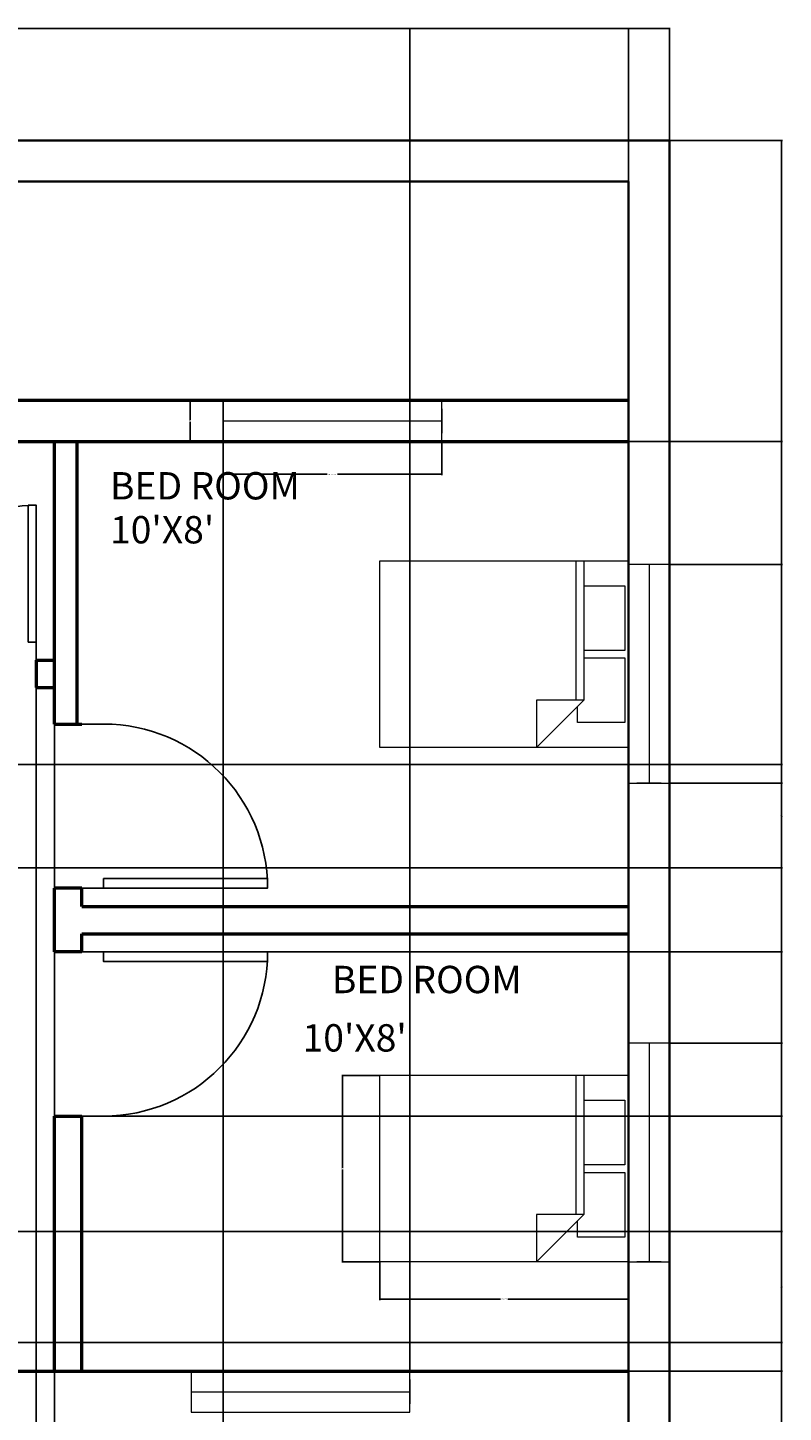
# Model space of a CAD drawing. Units: inches. Extents: x 8049 to 8459, y 820 to 1350.
# Tile 25 of 25: x 8294 to 8459, y 1046 to 1350. Entities that reach past the tile are written whole.
import ezdxf

# ---------------------------------------------------------------- set-up
doc = ezdxf.new("R2010")
doc.units = ezdxf.units.IN
doc.header["$MEASUREMENT"] = 0
for name, color, linetype, lineweight in [('A-ANNO-DIMS', 2, 'Continuous', 18), ('A-AREA-IDEN', 7, 'Continuous', 25), ('A-DOOR', 3, 'Continuous', 25), ('A-FURN', 8, 'Continuous', 18), ('A-GLAZ', 4, 'Continuous', 18), ('A-WALL', 7, 'Continuous', 50), ('C-SITE-WALL', 7, 'Continuous', 35)]:
    doc.layers.add(name, color=color, linetype=linetype, lineweight=lineweight)
doc.styles.get("Standard").update_dxf_attribs({"font": 'arial.ttf'})
doc.dimstyles.get("Standard").update_dxf_attribs({"dimtxt": 0.18, "dimasz": 0.18, "dimexe": 0.18, "dimexo": 0.0625, "dimgap": 0.09, "dimtad": 0, "dimtih": 1, "dimtoh": 1, "dimdec": 4, "dimzin": 0, "dimdsep": 46, "dimtxsty": 'Standard', "dimcen": 0.09, "dimadec": 0, "dimazin": 0, "dimtfac": 1, "dimtdec": 4, "dimtofl": 0, "dimtmove": 0, "dimatfit": 3, "dimfxl": 1, "dimtolj": 1, "dimtzin": 0, "dimarcsym": 0})

# ---------------------------------------------------------------- blocks, each defined once
blk = doc.blocks.new('*U2')
for p, q in [((0, 0), (0, -100)), ((750, 0), (750, -100))]:
    blk.add_line(p, q)
blk.add_lwpolyline([(0, 0), (0, 750), (43.75, 750), (43.75, 0)], close=True)
blk.add_arc((0, 0), 750, 0, 90)
blk = doc.blocks.new('*U4')
for p, q in [((0, 100), (0, 0)), ((900, 100), (900, 0)), ((0, 50), (900, 50))]:
    blk.add_line(p, q)
blk = doc.blocks.new('Bed - Queen')
for p, q in [((0, -80.00003), (0, 0)), ((0, 0), (59.99999, 0)), ((59.99999, 0), (59.99999, -80.00003)), ((7.99999, -1.2), (28.79998, -1.2)), ((7.99999, -14.4), (7.99999, -1.2)), ((28.79998, -1.2), (28.79998, -14.4)), ((31.19999, -1.2), (51.99999, -1.2)), ((31.19999, -14.4), (31.19999, -1.2)), ((51.99999, -1.2), (51.99999, -16.4)), ((0, -14.4), (44.8, -14.4)), ((44.8, -16.8), (0, -16.8)), ((59.99999, -29.6), (44.8, -14.4)), ((44.8, -14.4), (44.8, -29.6)), ((51.99999, -16.4), (46.79936, -16.4)), ((44.8, -29.6), (59.99999, -29.6)), ((59.99999, -80.00003), (0, -80.00003))]:
    blk.add_line(p, q)
blk = doc.blocks.new('WIN-48IN-SURROUND')
for p, q in [((9, 48), (0, 48)), ((0, 48), (0, 0)), ((0, 0), (9, 0))]:
    blk.add_line(p, q)
blk = doc.blocks.new('*D30')
at = {"layer": 'A-ANNO-DIMS', "color": 0, "lineweight": -2, "transparency": 16777216}
for p, q in [((8336.4, 1258.81), (8336.4, 1251.49)), ((8384.4, 1258.81), (8384.4, 1251.49)), ((8336.58, 1251.67), (8359.28, 1251.67)), ((8384.22, 1251.67), (8361.52, 1251.67))]:
    blk.add_line(p, q, dxfattribs=at)
at = {"layer": 'A-ANNO-DIMS', "color": 0, "transparency": 16777216}
for points in [[(8336.58, 1251.7), (8336.58, 1251.64), (8336.4, 1251.67)], [(8384.22, 1251.7), (8384.22, 1251.64), (8384.4, 1251.67)]]:
    blk.add_solid(points, dxfattribs=at)
at = {"layer": 'Defpoints', "color": 0, "transparency": 16777216}
for p in [(8336.4, 1258.87), (8384.4, 1258.87), (8384.4, 1251.67)]:
    blk.add_point(p, dxfattribs=at)
at = {"layer": 'A-ANNO-DIMS', "color": 0, "transparency": 16777216, "insert": (8360.4, 1251.67), "char_height": 0.18, "attachment_point": 5}
blk.add_mtext('\\A1;WINDOW 48 TYP.', dxfattribs=at)
blk = doc.blocks.new('*D31')
at = {"layer": 'A-ANNO-DIMS', "color": 0, "lineweight": -2, "transparency": 16777216}
for p, q in [((8336.33, 1267.87), (8329.02, 1267.87)), ((8329.2, 1267.69), (8329.2, 1263.55)), ((8329.2, 1259.05), (8329.2, 1263.19)), ((8336.33, 1258.87), (8329.02, 1258.87))]:
    blk.add_line(p, q, dxfattribs=at)
at = {"layer": 'A-ANNO-DIMS', "color": 0, "transparency": 16777216}
for points in [[(8329.17, 1267.69), (8329.23, 1267.69), (8329.2, 1267.87)], [(8329.17, 1259.05), (8329.23, 1259.05), (8329.2, 1258.87)]]:
    blk.add_solid(points, dxfattribs=at)
at = {"layer": 'Defpoints', "color": 0, "transparency": 16777216}
for p in [(8336.4, 1267.87), (8329.2, 1258.87), (8336.4, 1258.87)]:
    blk.add_point(p, dxfattribs=at)
at = {"layer": 'A-ANNO-DIMS', "color": 0, "transparency": 16777216, "insert": (8329.2, 1263.37), "char_height": 0.18, "attachment_point": 5}
blk.add_mtext('\\A1;9 TYP.', dxfattribs=at)
blk = doc.blocks.new('*D34')
at = {"layer": 'A-ANNO-DIMS', "color": 0, "lineweight": -2, "transparency": 16777216}
for p, q in [((8370.82, 1078.81), (8370.82, 1070.5)), ((8425.4, 1078.81), (8425.4, 1070.5)), ((8371, 1070.68), (8397.29, 1070.68)), ((8425.22, 1070.68), (8398.93, 1070.68))]:
    blk.add_line(p, q, dxfattribs=at)
at = {"layer": 'A-ANNO-DIMS', "color": 0, "transparency": 16777216}
for points in [[(8371, 1070.71), (8371, 1070.65), (8370.82, 1070.68)], [(8425.22, 1070.71), (8425.22, 1070.65), (8425.4, 1070.68)]]:
    blk.add_solid(points, dxfattribs=at)
at = {"layer": 'Defpoints', "color": 0, "transparency": 16777216}
for p in [(8370.82, 1078.87), (8425.4, 1078.87), (8425.4, 1070.68)]:
    blk.add_point(p, dxfattribs=at)
at = {"layer": 'A-ANNO-DIMS', "color": 0, "transparency": 16777216, "insert": (8398.11, 1070.68), "char_height": 0.18, "attachment_point": 5}
blk.add_mtext('\\A1;BED 55 TYP.', dxfattribs=at)
blk = doc.blocks.new('*D35')
at = {"layer": 'A-ANNO-DIMS', "color": 0, "lineweight": -2, "transparency": 16777216}
for p, q in [((8370.76, 1119.8), (8362.46, 1119.8)), ((8362.64, 1119.62), (8362.64, 1099.52)), ((8362.64, 1079.05), (8362.64, 1099.16)), ((8370.76, 1078.87), (8362.46, 1078.87))]:
    blk.add_line(p, q, dxfattribs=at)
at = {"layer": 'A-ANNO-DIMS', "color": 0, "transparency": 16777216}
for points in [[(8362.61, 1119.62), (8362.67, 1119.62), (8362.64, 1119.8)], [(8362.61, 1079.05), (8362.67, 1079.05), (8362.64, 1078.87)]]:
    blk.add_solid(points, dxfattribs=at)
at = {"layer": 'Defpoints', "color": 0, "transparency": 16777216}
for p in [(8370.82, 1119.8), (8362.64, 1078.87), (8370.82, 1078.87)]:
    blk.add_point(p, dxfattribs=at)
at = {"layer": 'A-ANNO-DIMS', "color": 0, "transparency": 16777216, "insert": (8362.64, 1099.34), "char_height": 0.18, "attachment_point": 5}
blk.add_mtext('\\A1;41 TYP.', dxfattribs=at)
blk = doc.blocks.new('*D48')
at = {"layer": 'A-ANNO-DIMS', "color": 0, "lineweight": -2, "transparency": 16777216}
for p, q in [((8074.4, 1324.93), (8074.4, 1349.65)), ((8074.58, 1349.47), (8254.11, 1349.47)), ((8434.22, 1349.47), (8254.69, 1349.47)), ((8434.4, 1324.93), (8434.4, 1349.65))]:
    blk.add_line(p, q, dxfattribs=at)
at = {"layer": 'A-ANNO-DIMS', "color": 0, "transparency": 16777216}
for points in [[(8074.58, 1349.5), (8074.58, 1349.44), (8074.4, 1349.47)], [(8434.22, 1349.5), (8434.22, 1349.44), (8434.4, 1349.47)]]:
    blk.add_solid(points, dxfattribs=at)
at = {"layer": 'Defpoints', "color": 0, "transparency": 16777216}
for p in [(8434.4, 1349.47), (8074.4, 1324.87), (8434.4, 1324.87)]:
    blk.add_point(p, dxfattribs=at)
at = {"layer": 'A-ANNO-DIMS', "color": 0, "transparency": 16777216, "insert": (8254.4, 1349.47), "char_height": 0.18, "attachment_point": 5}
blk.add_mtext('\\A1;360', dxfattribs=at)
blk = doc.blocks.new('*D49')
at = {"layer": 'A-ANNO-DIMS', "color": 0, "lineweight": -2, "transparency": 16777216}
for p, q in [((8434.46, 1324.87), (8459.18, 1324.87)), ((8459, 1324.69), (8459, 1085.05)), ((8459, 845.05), (8459, 1084.69)), ((8434.46, 844.87), (8459.18, 844.87))]:
    blk.add_line(p, q, dxfattribs=at)
at = {"layer": 'A-ANNO-DIMS', "color": 0, "transparency": 16777216}
for points in [[(8458.97, 1324.69), (8459.03, 1324.69), (8459, 1324.87)], [(8458.97, 845.05), (8459.03, 845.05), (8459, 844.87)]]:
    blk.add_solid(points, dxfattribs=at)
at = {"layer": 'Defpoints', "color": 0, "transparency": 16777216}
for p in [(8434.4, 1324.87), (8459, 1324.87), (8434.4, 844.87)]:
    blk.add_point(p, dxfattribs=at)
at = {"layer": 'A-ANNO-DIMS', "color": 0, "transparency": 16777216, "insert": (8459, 1084.87), "char_height": 0.18, "attachment_point": 5}
blk.add_mtext('\\A1;480', dxfattribs=at)
blk = doc.blocks.new('*D66')
at = {"layer": 'A-ANNO-DIMS', "color": 0, "lineweight": -2, "transparency": 16777216}
for p, q in [((8336.4, 1267.81), (8336.4, 820.09)), ((8299.4, 1258.81), (8299.4, 820.09)), ((8299.58, 820.27), (8317.68, 820.27)), ((8336.22, 820.27), (8318.12, 820.27))]:
    blk.add_line(p, q, dxfattribs=at)
at = {"layer": 'A-ANNO-DIMS', "color": 0, "transparency": 16777216}
for points in [[(8299.58, 820.3), (8299.58, 820.24), (8299.4, 820.27)], [(8336.22, 820.3), (8336.22, 820.24), (8336.4, 820.27)]]:
    blk.add_solid(points, dxfattribs=at)
at = {"layer": 'Defpoints', "color": 0, "transparency": 16777216}
for p in [(8336.4, 1267.87), (8299.4, 1258.87), (8299.4, 820.27)]:
    blk.add_point(p, dxfattribs=at)
at = {"layer": 'A-ANNO-DIMS', "color": 0, "transparency": 16777216, "insert": (8317.9, 820.27), "char_height": 0.18, "attachment_point": 5}
blk.add_mtext('\\A1;37', dxfattribs=at)
blk = doc.blocks.new('*D67')
at = {"layer": 'A-ANNO-DIMS', "color": 0, "lineweight": -2, "transparency": 16777216}
for p, q in [((8425.46, 1258.87), (8459.18, 1258.87)), ((8459, 1258.69), (8459, 1245.55)), ((8459, 1232.05), (8459, 1245.19)), ((8434.46, 1231.87), (8459.18, 1231.87))]:
    blk.add_line(p, q, dxfattribs=at)
at = {"layer": 'A-ANNO-DIMS', "color": 0, "transparency": 16777216}
for points in [[(8458.97, 1258.69), (8459.03, 1258.69), (8459, 1258.87)], [(8458.97, 1232.05), (8459.03, 1232.05), (8459, 1231.87)]]:
    blk.add_solid(points, dxfattribs=at)
at = {"layer": 'Defpoints', "color": 0, "transparency": 16777216}
for p in [(8425.4, 1258.87), (8459, 1258.87), (8434.4, 1231.87)]:
    blk.add_point(p, dxfattribs=at)
at = {"layer": 'A-ANNO-DIMS', "color": 0, "transparency": 16777216, "insert": (8459, 1245.37), "char_height": 0.18, "attachment_point": 5}
blk.add_mtext('\\A1;27', dxfattribs=at)
blk = doc.blocks.new('*D68')
at = {"layer": 'A-ANNO-DIMS', "color": 0, "lineweight": -2, "transparency": 16777216}
for p, q in [((8434.46, 1183.87), (8459.18, 1183.87)), ((8459, 1183.69), (8459, 1155.55)), ((8459, 1127.05), (8459, 1155.19)), ((8434.46, 1126.87), (8459.18, 1126.87))]:
    blk.add_line(p, q, dxfattribs=at)
at = {"layer": 'A-ANNO-DIMS', "color": 0, "transparency": 16777216}
for points in [[(8458.97, 1183.69), (8459.03, 1183.69), (8459, 1183.87)], [(8458.97, 1127.05), (8459.03, 1127.05), (8459, 1126.87)]]:
    blk.add_solid(points, dxfattribs=at)
at = {"layer": 'Defpoints', "color": 0, "transparency": 16777216}
for p in [(8434.4, 1183.87), (8459, 1183.87), (8434.4, 1126.87)]:
    blk.add_point(p, dxfattribs=at)
at = {"layer": 'A-ANNO-DIMS', "color": 0, "transparency": 16777216, "insert": (8459, 1155.37), "char_height": 0.18, "attachment_point": 5}
blk.add_mtext('\\A1;57', dxfattribs=at)
blk = doc.blocks.new('*D69')
at = {"layer": 'A-ANNO-DIMS', "color": 0, "lineweight": -2, "transparency": 16777216}
for p, q in [((8377.4, 1054.93), (8377.4, 1349.65)), ((8377.58, 1349.47), (8401.17, 1349.47)), ((8425.22, 1349.47), (8401.62, 1349.47)), ((8425.4, 1054.93), (8425.4, 1349.65))]:
    blk.add_line(p, q, dxfattribs=at)
at = {"layer": 'A-ANNO-DIMS', "color": 0, "transparency": 16777216}
for points in [[(8377.58, 1349.5), (8377.58, 1349.44), (8377.4, 1349.47)], [(8425.22, 1349.5), (8425.22, 1349.44), (8425.4, 1349.47)]]:
    blk.add_solid(points, dxfattribs=at)
at = {"layer": 'Defpoints', "color": 0, "transparency": 16777216}
for p in [(8377.4, 1349.47), (8377.4, 1054.87), (8425.4, 1054.87)]:
    blk.add_point(p, dxfattribs=at)
at = {"layer": 'A-ANNO-DIMS', "color": 0, "transparency": 16777216, "insert": (8401.4, 1349.47), "char_height": 0.18, "attachment_point": 5}
blk.add_mtext('\\A1;48', dxfattribs=at)
blk = doc.blocks.new('*D74')
at = {"layer": 'A-ANNO-DIMS', "color": 0, "lineweight": -2, "transparency": 16777216}
for p, q in [((8299.46, 1146.87), (8459.18, 1146.87)), ((8459, 1146.69), (8459, 1129.05)), ((8459, 1111.05), (8459, 1128.69)), ((8299.46, 1110.87), (8459.18, 1110.87))]:
    blk.add_line(p, q, dxfattribs=at)
at = {"layer": 'A-ANNO-DIMS', "color": 0, "transparency": 16777216}
for points in [[(8458.97, 1146.69), (8459.03, 1146.69), (8459, 1146.87)], [(8458.97, 1111.05), (8459.03, 1111.05), (8459, 1110.87)]]:
    blk.add_solid(points, dxfattribs=at)
at = {"layer": 'Defpoints', "color": 0, "transparency": 16777216}
for p in [(8299.4, 1146.87), (8459, 1146.87), (8299.4, 1110.87)]:
    blk.add_point(p, dxfattribs=at)
at = {"layer": 'A-ANNO-DIMS', "color": 0, "transparency": 16777216, "insert": (8459, 1128.87), "char_height": 0.18, "attachment_point": 5}
blk.add_mtext('\\A1;36', dxfattribs=at)
blk = doc.blocks.new('*D76')
at = {"layer": 'A-ANNO-DIMS', "color": 0, "lineweight": -2, "transparency": 16777216}
for p, q in [((8083.4, 1054.81), (8083.4, 820.09)), ((8299.4, 1054.81), (8299.4, 820.09)), ((8083.58, 820.27), (8191.11, 820.27)), ((8299.22, 820.27), (8191.69, 820.27))]:
    blk.add_line(p, q, dxfattribs=at)
at = {"layer": 'A-ANNO-DIMS', "color": 0, "transparency": 16777216}
for points in [[(8083.58, 820.3), (8083.58, 820.24), (8083.4, 820.27)], [(8299.22, 820.3), (8299.22, 820.24), (8299.4, 820.27)]]:
    blk.add_solid(points, dxfattribs=at)
at = {"layer": 'Defpoints', "color": 0, "transparency": 16777216}
for p in [(8083.4, 1054.87), (8299.4, 1054.87), (8299.4, 820.27)]:
    blk.add_point(p, dxfattribs=at)
at = {"layer": 'A-ANNO-DIMS', "color": 0, "transparency": 16777216, "insert": (8191.4, 820.27), "char_height": 0.18, "attachment_point": 5}
blk.add_mtext('\\A1;216', dxfattribs=at)
blk = doc.blocks.new('*D80')
at = {"layer": 'A-ANNO-DIMS', "color": 0, "lineweight": -2, "transparency": 16777216}
for p, q in [((8206.43, 1085.56), (8459.18, 1085.56)), ((8459, 1085.38), (8459, 1073.55)), ((8459, 1061.35), (8459, 1073.19)), ((8206.43, 1061.17), (8459.18, 1061.17))]:
    blk.add_line(p, q, dxfattribs=at)
at = {"layer": 'A-ANNO-DIMS', "color": 0, "transparency": 16777216}
for points in [[(8458.97, 1085.38), (8459.03, 1085.38), (8459, 1085.56)], [(8458.97, 1061.35), (8459.03, 1061.35), (8459, 1061.17)]]:
    blk.add_solid(points, dxfattribs=at)
at = {"layer": 'Defpoints', "color": 0, "transparency": 16777216}
for p in [(8206.37, 1085.56), (8459, 1085.56), (8206.37, 1061.17)]:
    blk.add_point(p, dxfattribs=at)
at = {"layer": 'A-ANNO-DIMS', "color": 0, "transparency": 16777216, "insert": (8459, 1073.37), "char_height": 0.18, "attachment_point": 5}
blk.add_mtext('\\A1;24.386', dxfattribs=at)
blk = doc.blocks.new('*D81')
at = {"layer": 'A-ANNO-DIMS', "color": 0, "lineweight": -2, "transparency": 16777216}
for p, q in [((8299.46, 1110.87), (8459.18, 1110.87)), ((8459, 1110.69), (8459, 1083.05)), ((8459, 1055.05), (8459, 1082.69)), ((8299.46, 1054.87), (8459.18, 1054.87))]:
    blk.add_line(p, q, dxfattribs=at)
at = {"layer": 'A-ANNO-DIMS', "color": 0, "transparency": 16777216}
for points in [[(8458.97, 1110.69), (8459.03, 1110.69), (8459, 1110.87)], [(8458.97, 1055.05), (8459.03, 1055.05), (8459, 1054.87)]]:
    blk.add_solid(points, dxfattribs=at)
at = {"layer": 'Defpoints', "color": 0, "transparency": 16777216}
for p in [(8299.4, 1110.87), (8459, 1110.87), (8299.4, 1054.87)]:
    blk.add_point(p, dxfattribs=at)
at = {"layer": 'A-ANNO-DIMS', "color": 0, "transparency": 16777216, "insert": (8459, 1082.87), "char_height": 0.18, "attachment_point": 5}
blk.add_mtext('\\A1;56', dxfattribs=at)
blk = doc.blocks.new('*D83')
at = {"layer": 'A-ANNO-DIMS', "color": 0, "lineweight": -2, "transparency": 16777216}
for p, q in [((8112.96, 1187.99), (8459.18, 1187.99)), ((8459, 1187.81), (8459, 1176.83)), ((8459, 1165.49), (8459, 1176.47)), ((8112.96, 1165.31), (8459.18, 1165.31))]:
    blk.add_line(p, q, dxfattribs=at)
at = {"layer": 'A-ANNO-DIMS', "color": 0, "transparency": 16777216}
for points in [[(8458.97, 1187.81), (8459.03, 1187.81), (8459, 1187.99)], [(8458.97, 1165.49), (8459.03, 1165.49), (8459, 1165.31)]]:
    blk.add_solid(points, dxfattribs=at)
at = {"layer": 'Defpoints', "color": 0, "transparency": 16777216}
for p in [(8112.9, 1187.99), (8459, 1187.99), (8112.9, 1165.31)]:
    blk.add_point(p, dxfattribs=at)
at = {"layer": 'A-ANNO-DIMS', "color": 0, "transparency": 16777216, "insert": (8459, 1176.65), "char_height": 0.18, "attachment_point": 5}
blk.add_mtext('\\A1;22.68', dxfattribs=at)
blk = doc.blocks.new('*D86')
at = {"layer": 'A-ANNO-DIMS', "color": 0, "lineweight": -2, "transparency": 16777216}
for p, q in [((8265.4, 1204.81), (8265.4, 820.09)), ((8295.4, 1204.81), (8295.4, 820.09)), ((8265.58, 820.27), (8280.18, 820.27)), ((8295.22, 820.27), (8280.62, 820.27))]:
    blk.add_line(p, q, dxfattribs=at)
at = {"layer": 'A-ANNO-DIMS', "color": 0, "transparency": 16777216}
for points in [[(8265.58, 820.3), (8265.58, 820.24), (8265.4, 820.27)], [(8295.22, 820.3), (8295.22, 820.24), (8295.4, 820.27)]]:
    blk.add_solid(points, dxfattribs=at)
at = {"layer": 'Defpoints', "color": 0, "transparency": 16777216}
for p in [(8265.4, 1204.87), (8295.4, 1204.87), (8295.4, 820.27)]:
    blk.add_point(p, dxfattribs=at)
at = {"layer": 'A-ANNO-DIMS', "color": 0, "transparency": 16777216, "insert": (8280.4, 820.27), "char_height": 0.18, "attachment_point": 5}
blk.add_mtext('\\A1;30', dxfattribs=at)

msp = doc.modelspace()

# ---------------------------------------------------------------- linework, layer by layer
at = {"layer": 'A-WALL'}
for p, q in [((8425.3974, 1267.8706), (8117.3974, 1267.8706)), ((8117.3974, 1258.8706), (8425.3974, 1258.8706)), ((8299.3974, 1196.8706), (8299.3974, 1258.8706)), ((8304.3974, 1196.8706), (8304.3974, 1258.8706)), ((8295.3974, 1210.8706), (8295.3974, 1204.8706)), ((8295.3974, 1210.8706), (8299.3974, 1210.8706)), ((8295.3974, 1204.8706), (8299.3974, 1204.8706)), ((8299.3974, 1196.8706), (8305.3974, 1196.8706)), ((8305.3974, 1160.8706), (8299.3974, 1160.8706)), ((8299.3974, 1146.8706), (8299.3974, 1160.8706)), ((8305.3974, 1156.8706), (8305.3974, 1160.8706)), ((8305.3974, 1156.8706), (8425.3974, 1156.8706)), ((8305.3974, 1150.8706), (8425.3974, 1150.8706)), ((8305.3974, 1146.8706), (8305.3974, 1150.8706)), ((8305.3974, 1146.8706), (8299.3974, 1146.8706)), ((8299.3974, 1054.8706), (8299.3974, 1110.8706)), ((8299.3974, 1110.8706), (8305.3974, 1110.8706)), ((8305.3974, 1054.8706), (8305.3974, 1110.8706)), ((8281.3974, 1054.8706), (8425.3974, 1054.8706))]:
    msp.add_line(p, q, dxfattribs=at)
at = {"layer": 'C-SITE-WALL'}
for p, q in [((8434.3974, 1324.8706), (8074.3974, 1324.8706)), ((8434.3974, 844.8706), (8434.3974, 1324.8706)), ((8425.3974, 1315.8706), (8083.3974, 1315.8706)), ((8425.3974, 853.8706), (8425.3974, 1315.8706))]:
    msp.add_line(p, q, dxfattribs=at)

# ---------------------------------------------------------------- block references
at = {"layer": 'A-DOOR', "xscale": -0.0399999999999999, "yscale": 0.0399999999999999, "zscale": 0.0399999999999999}
msp.add_blockref('*U2', (8295.3974, 1214.8706), dxfattribs=at)
at = {"layer": 'A-DOOR', "yscale": 0.0479999999999998, "zscale": 0.0479999999999998, "rotation": 270}
for p, xscale in [((8310.1974, 1160.8706), -0.0479999999999998), ((8310.1974, 1146.8706), 0.0479999999999998)]:
    msp.add_blockref('*U2', p, dxfattribs=dict(at, xscale=xscale))
at = {"layer": 'A-FURN', "xscale": 0.6821843913493107, "yscale": 0.6821843913493107, "zscale": 0.6821843913493107, "rotation": 270}
for p in [(8425.3974, 1232.6555), (8425.3974, 1119.8017)]:
    msp.add_blockref('Bed - Queen', p, dxfattribs=at)
at = {"layer": 'A-GLAZ'}
for p, rotation in [((8336.3978, 1267.871), 269.999999999998), ((8434.3978, 1231.8702), 180), ((8434.3978, 1126.8702), 180), ((8377.397, 1045.8702), 89.99999999999795)]:
    msp.add_blockref('WIN-48IN-SURROUND', p, dxfattribs=dict(at, rotation=rotation))
at = {"layer": 'A-GLAZ', "xscale": 0.0533333333333332, "yscale": 0.0533333333333332, "zscale": 0.0533333333333332}
for p in [(8336.3974, 1260.7039), (8329.3974, 1047.7039)]:
    msp.add_blockref('*U4', p, dxfattribs=at)
at = {"layer": 'A-GLAZ', "xscale": 0.0533333333333332, "yscale": 0.0533333333333332, "zscale": 0.0533333333333332, "rotation": 270}
for p in [(8427.2307, 1231.8706), (8427.2307, 1126.8706)]:
    msp.add_blockref('*U4', p, dxfattribs=at)

# ---------------------------------------------------------------- texts
at = {"layer": 'A-AREA-IDEN'}
for s, p in [('BED ROOM', (8311.5978, 1246.1461)), ("10'X8'", (8311.5978, 1236.5076)), ('BED ROOM', (8360.2919, 1137.827)), ("10'X8'", (8353.856, 1125.0243))]:
    msp.add_text(s, height=6, dxfattribs=at).set_placement(p)

# ---------------------------------------------------------------- dimensions: what is measured, and where the dimension line sits
at = {"layer": 'A-ANNO-DIMS'}
for base, p1, p2, picture, middle in [((8434.3974, 1349.4706), (8074.3974, 1324.8706), (8434.3974, 1324.8706), '*D48', (8254.3974, 1349.4706)), ((8377.3974, 1349.4706), (8425.3974, 1054.8706), (8377.3974, 1054.8706), '*D69', (8401.3974, 1349.4706)), ((8299.3974, 820.2706), (8336.3974, 1267.8706), (8299.3974, 1258.8706), '*D66', (8317.8974, 820.2706)), ((8295.3974, 820.2706), (8265.3974, 1204.8706), (8295.3974, 1204.8706), '*D86', (8280.3974, 820.2706)), ((8299.3974, 820.2706), (8083.3974, 1054.8706), (8299.3974, 1054.8706), '*D76', (8191.3974, 820.2706))]:
    dim = msp.add_linear_dim(base=base, p1=p1, p2=p2, dimstyle='Standard', override={"dimdec": 0, "dimlfac": 1, "dimrnd": 0, "dimzin": 0, "dimdsep": 46, "dimlunit": 2}, dxfattribs=at)
    dim.commit()
    dim.dimension.update_dxf_attribs({"geometry": picture, "text_midpoint": middle})
for base, p1, p2, override, picture, middle in [((8458.9974, 1324.8706), (8434.3974, 844.8706), (8434.3974, 1324.8706), {"dimdec": 0, "dimlfac": 1, "dimrnd": 0, "dimzin": 0, "dimdsep": 46, "dimlunit": 2}, '*D49', (8458.9974, 1084.8706)), ((8458.9974, 1258.8706), (8434.3974, 1231.8706), (8425.3974, 1258.8706), {"dimdec": 0, "dimlfac": 1, "dimrnd": 0, "dimzin": 0, "dimdsep": 46, "dimlunit": 2}, '*D67', (8458.9974, 1245.3706)), ((8458.9974, 1187.9939), (8112.9001, 1165.3117), (8112.9001, 1187.9939), {"dimdec": 2, "dimlfac": 1, "dimrnd": 0, "dimzin": 0, "dimdsep": 46, "dimlunit": 2}, '*D83', (8458.9974, 1176.6528)), ((8458.9974, 1183.8706), (8434.3974, 1126.8706), (8434.3974, 1183.8706), {"dimdec": 0, "dimlfac": 1, "dimrnd": 0, "dimzin": 0, "dimdsep": 46, "dimlunit": 2}, '*D68', (8458.9974, 1155.3706)), ((8458.9974, 1146.8706), (8299.3974, 1110.8706), (8299.3974, 1146.8706), {"dimdec": 0, "dimlfac": 1, "dimrnd": 0, "dimzin": 0, "dimdsep": 46, "dimlunit": 2}, '*D74', (8458.9974, 1128.8706)), ((8458.9974, 1110.8706), (8299.3974, 1054.8706), (8299.3974, 1110.8706), {"dimdec": 0, "dimlfac": 1, "dimrnd": 0, "dimzin": 0, "dimdsep": 46, "dimlunit": 2}, '*D81', (8458.9974, 1082.8706)), ((8458.9974, 1085.5602), (8206.3663, 1061.1739), (8206.3663, 1085.5602), {"dimdec": 3, "dimlfac": 1, "dimrnd": 0, "dimzin": 0, "dimdsep": 46, "dimlunit": 2}, '*D80', (8458.9974, 1073.3671))]:
    dim = msp.add_linear_dim(base=base, p1=p1, p2=p2, angle=90, dimstyle='Standard', override=override, dxfattribs=at)
    dim.commit()
    dim.dimension.update_dxf_attribs({"geometry": picture, "text_midpoint": middle})
for base, p1, p2, picture, middle in [((8329.1974, 1258.8706), (8336.3974, 1267.8706), (8336.3974, 1258.8706), '*D31', (8329.1974, 1263.3706)), ((8362.6364, 1078.8706), (8370.8226, 1119.8017), (8370.8226, 1078.8706), '*D35', (8362.6364, 1099.3361))]:
    dim = msp.add_linear_dim(base=base, p1=p1, p2=p2, angle=270, text='<> TYP.', dimstyle='Standard', override={"dimdec": 0, "dimlfac": 1, "dimrnd": 0, "dimzin": 0, "dimdsep": 46, "dimlunit": 2}, dxfattribs=at)
    dim.commit()
    dim.dimension.update_dxf_attribs({"geometry": picture, "text_midpoint": middle})
for base, p1, p2, text, picture, middle in [((8384.3974, 1251.6706), (8336.3974, 1258.8706), (8384.3974, 1258.8706), 'WINDOW <> TYP.', '*D30', (8360.3974, 1251.6706)), ((8425.3974, 1070.6844), (8370.8226, 1078.8706), (8425.3974, 1078.8706), 'BED <> TYP.', '*D34', (8398.11, 1070.6844))]:
    dim = msp.add_linear_dim(base=base, p1=p1, p2=p2, text=text, dimstyle='Standard', override={"dimdec": 0, "dimlfac": 1, "dimrnd": 0, "dimzin": 0, "dimdsep": 46, "dimlunit": 2}, dxfattribs=at)
    dim.commit()
    dim.dimension.update_dxf_attribs({"geometry": picture, "text_midpoint": middle})

doc.saveas('drawing.dxf')
